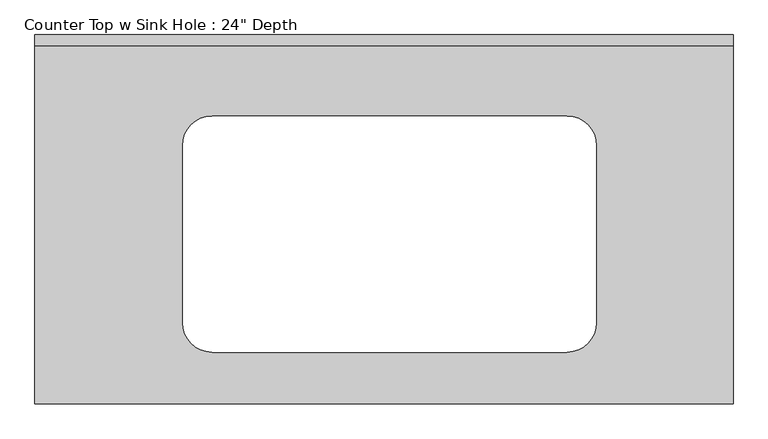
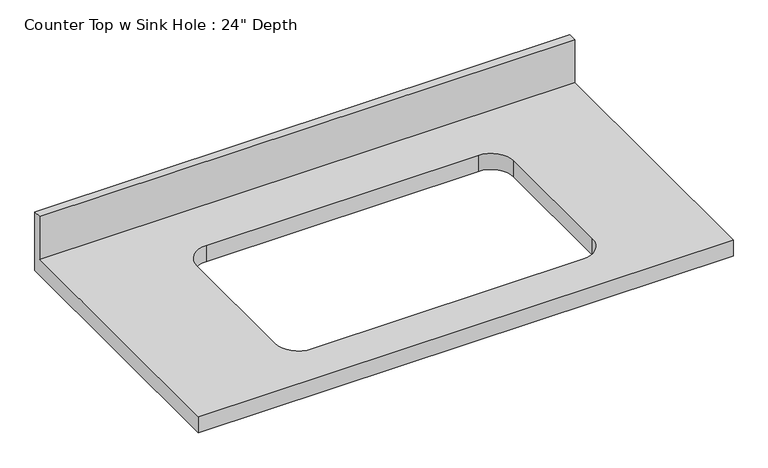
"""IFC4 building model written with IfcOpenShell, lengths in millimetres: furniture geometry."""

from ifc_helpers import new_model, si_unit, frame, origin, place, context, project, spatial, polyline, circle_curve, source, transform, mapped, element, save
from ifc_brep_helpers import plane_surface, revolved_surface, advanced_brep


def furniture_8d0dc8c9(model_context):
    return source(origin(), model_context, "Body", "AdvancedBrep", [
        advanced_brep(
        [(-1200.4622951, -635.0, 914.4), (-0.130724, -635.0, 914.4), (-0.130724, -19.05, 914.4), (-1200.4622951, -19.05, 914.4), (-895.6622951, -139.7, 914.4), (-286.0622951, -139.7, 914.4), (-235.2622951, -190.5, 914.4), (-235.2622951, -495.3, 914.4), (-286.0622951, -546.1, 914.4), (-895.6622951, -546.1, 914.4), (-946.4622951, -495.3, 914.4), (-946.4622951, -190.5, 914.4), (-0.130724, 0.0, 876.3), (-0.130724, -635.0, 876.3), (-1200.4622951, -635.0, 876.3), (-1200.4622951, 0.0, 876.3), (-286.0622951, -139.7, 876.3), (-895.6622951, -139.7, 876.3), (-946.4622951, -190.5, 876.3), (-946.4622951, -495.3, 876.3), (-895.6622951, -546.1, 876.3), (-286.0622951, -546.1, 876.3), (-235.2622951, -495.3, 876.3), (-235.2622951, -190.5, 876.3), (-1200.4622951, 0.0, 1016.0), (-0.130724, 0.0, 1016.0), (-1200.4622951, -19.05, 1016.0), (-0.130724, -19.05, 1016.0)],
        [
            (0, 1),
            (1, 2),
            (2, 3),
            (3, 0),
            (4, 5),
            (5, 6, circle_curve(frame((-286.0622951, -190.5, 914.4), z_axis=(0.0, 0.0, -1.0), x_axis=(1.0, 0.0, 0.0)), 50.8)),
            (6, 7),
            (7, 8, circle_curve(frame((-286.0622951, -495.3, 914.4), z_axis=(0.0, 0.0, -1.0), x_axis=(1.0, 0.0, 0.0)), 50.8)),
            (8, 9),
            (9, 10, circle_curve(frame((-895.6622951, -495.3, 914.4), z_axis=(0.0, 0.0, -1.0), x_axis=(1.0, 0.0, 0.0)), 50.8)),
            (10, 11),
            (11, 4, circle_curve(frame((-895.6622951, -190.5, 914.4), z_axis=(0.0, 0.0, -1.0), x_axis=(1.0, 0.0, 0.0)), 50.8)),
            (12, 13),
            (13, 14),
            (14, 15),
            (15, 12),
            (16, 17),
            (17, 18, circle_curve(frame((-895.6622951, -190.5, 876.3), z_axis=(0.0, 0.0, 1.0), x_axis=(1.0, 0.0, 0.0)), 50.8)),
            (18, 19),
            (19, 20, circle_curve(frame((-895.6622951, -495.3, 876.3), z_axis=(0.0, 0.0, 1.0), x_axis=(1.0, 0.0, 0.0)), 50.8)),
            (20, 21),
            (21, 22, circle_curve(frame((-286.0622951, -495.3, 876.3), z_axis=(0.0, 0.0, 1.0), x_axis=(1.0, 0.0, 0.0)), 50.8)),
            (22, 23),
            (23, 16, circle_curve(frame((-286.0622951, -190.5, 876.3), z_axis=(0.0, 0.0, 1.0), x_axis=(1.0, 0.0, 0.0)), 50.8)),
            (15, 24),
            (24, 25),
            (25, 12),
            (14, 0),
            (3, 26),
            (26, 24),
            (13, 1),
            (25, 27),
            (27, 2),
            (26, 27),
            (4, 17),
            (16, 5),
            (11, 18),
            (10, 19),
            (9, 20),
            (8, 21),
            (7, 22),
            (6, 23),
        ],
        [
            plane_surface(frame((-1200.4622951, 0.0, 914.4), z_axis=(0.0, 0.0, 1.0), x_axis=(-1.0, 0.0, 0.0))),
            plane_surface(frame((-1200.4622951, 0.0, 876.3), z_axis=(0.0, 0.0, -1.0), x_axis=(1.0, 0.0, 0.0))),
            plane_surface(frame((-0.130724, 0.0, 914.4), z_axis=(0.0, 1.0, 0.0), x_axis=(0.0, 0.0, -1.0))),
            plane_surface(frame((-1200.4622951, 0.0, 914.4), z_axis=(-1.0, 0.0, 0.0), x_axis=(0.0, 0.0, -1.0))),
            plane_surface(frame((-1200.4622951, -635.0, 914.4), z_axis=(0.0, -1.0, 0.0), x_axis=(0.0, 0.0, -1.0))),
            plane_surface(frame((-0.130724, -635.0, 914.4), z_axis=(1.0, 0.0, 0.0), x_axis=(0.0, 0.0, -1.0))),
            plane_surface(frame((-1200.4622951, 0.0, 1016.0), z_axis=(0.0, 0.0, 1.0), x_axis=(0.0, -1.0, 0.0))),
            plane_surface(frame((-1200.4622951, -19.05, 1016.0), z_axis=(0.0, -1.0, 0.0), x_axis=(0.0, 0.0, -1.0))),
            plane_surface(frame((-286.0622951, -139.7, 914.4), z_axis=(0.0, -1.0, 0.0), x_axis=(0.0, 0.0, -1.0))),
            revolved_surface(polyline([(-844.8622951000001, -190.5, 914.4), (-844.8622951000001, -190.5, 876.3)]), (-895.6622951, -190.5, 876.3), (0.0, 0.0, 1.0)),
            plane_surface(frame((-946.4622951, -190.5, 914.4), z_axis=(1.0, 0.0, 0.0), x_axis=(0.0, 0.0, -1.0))),
            revolved_surface(polyline([(-844.8622951000001, -495.3, 914.4), (-844.8622951000001, -495.3, 876.3)]), (-895.6622951, -495.3, 876.3), (0.0, 0.0, 1.0)),
            plane_surface(frame((-895.6622951, -546.1, 914.4), z_axis=(0.0, 1.0, 0.0), x_axis=(0.0, 0.0, -1.0))),
            revolved_surface(polyline([(-235.26229509999996, -495.3, 914.4), (-235.26229509999996, -495.3, 876.3)]), (-286.0622951, -495.3, 876.3), (0.0, 0.0, 1.0)),
            plane_surface(frame((-235.2622951, -495.3, 914.4), z_axis=(-1.0, 0.0, 0.0), x_axis=(0.0, 0.0, -1.0))),
            revolved_surface(polyline([(-235.26229509999996, -190.5, 914.4), (-235.26229509999996, -190.5, 876.3)]), (-286.0622951, -190.5, 876.3), (0.0, 0.0, 1.0)),
        ],
        [
            (0, [[1, 2, 3, 4], [5, 6, 7, 8, 9, 10, 11, 12]]),
            (1, [[13, 14, 15, 16], [17, 18, 19, 20, 21, 22, 23, 24]]),
            (2, [[-16, 25, 26, 27]]),
            (3, [[-15, 28, -4, 29, 30, -25]]),
            (4, [[-1, -28, -14, 31]]),
            (5, [[-13, -27, 32, 33, -2, -31]]),
            (6, [[-30, 34, -32, -26]]),
            (7, [[-34, -29, -3, -33]]),
            (8, [[35, -17, 36, -5]]),
            (9, [[-35, -12, 37, -18]]),
            (10, [[-37, -11, 38, -19]]),
            (11, [[-38, -10, 39, -20]]),
            (12, [[-39, -9, 40, -21]]),
            (13, [[-40, -8, 41, -22]]),
            (14, [[-41, -7, 42, -23]]),
            (15, [[-36, -24, -42, -6]]),
        ],
    ),
    ])


if __name__ == "__main__":
    model = new_model("IFC4")
    model_context = context("Model", 3, world=origin())
    ifc_project = project(units=[si_unit("LENGTHUNIT", "METRE", prefix="MILLI")], contexts=[model_context])
    site = spatial("IfcSite", under=ifc_project)
    building = spatial("IfcBuilding", under=site)
    placement = place(None, origin())
    furniture_shape = furniture_8d0dc8c9(model_context)
    element("IfcFurniture", 1, ObjectType="Counter Top w Sink Hole : 24\" Depth", at=placement, inside=building, context=model_context, shape_type="MappedRepresentation", body=[
        mapped(furniture_shape, transform((0.0, 0.0, 0.0), x_axis=(1.0, 0.0, 0.0), y_axis=(0.0, 1.0, 0.0), z_axis=(0.0, 0.0, 1.0))),
    ])
    save(model, "model.ifc")

# Revit data of these elements
# Type "Counter Top w Sink Hole : 24\" Depth"
#   Assembly Code = "C1030400"
#   Counter Thickness = 0' - 1 1/2"
#   Depth = 2' - 1"
#   Height = 3' - 0"
#   Length [instance default] = 8' - 0"
#   Sink Location [instance default] = 2' - 0"
#   Sink Location To Wall [instance default] = 0' - 6"
#   Sink Opening Depth [instance default] = 1' - 3"
#   Sink Opening Width [instance default] = 2' - 3"
#   Counter Top Material = none
#   Default Elevation = 0
# Element 1 (IfcFurniture, "Counter Top w Sink Hole : 24\" Depth")
#   Length = 3' - 11.25715"
#   Materials on its faces: "Counter Top"
# Materials
#   "Counter Top": class "Wood", colour RGB 226 177 128, transparency 0
